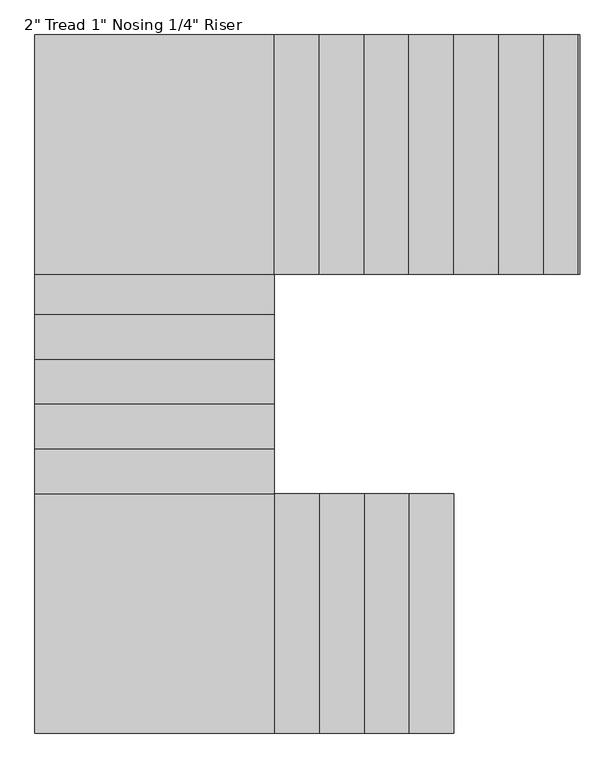
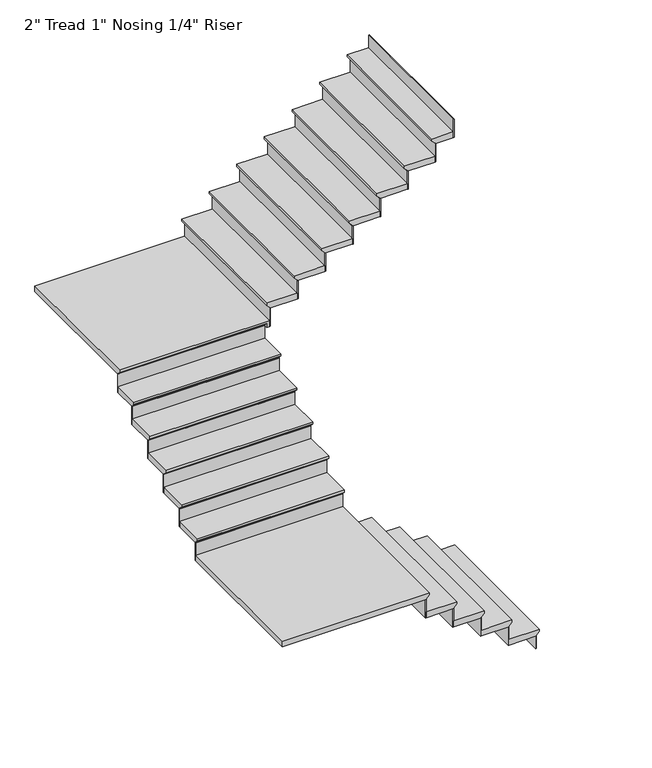
"""IFC4 building model written with IfcOpenShell, lengths in millimetres: stair flight geometry."""

from ifc_helpers import new_model, si_unit, origin, place, context, project, spatial, faceted_brep, source, transform, mapped, element, save


def stair_flight_7559bbc3(model_context):
    return source(origin(), model_context, "Body", "Brep", [
        faceted_brep([(-2683.1105391, -1521.8373761, 3189.3710526), (-2683.1105391, -1521.8373761, 3208.4210526), (-2683.1105391, -2741.0373761, 3208.4210526), (-2683.1105391, -2741.0373761, 3189.3710526), (-2708.5105391, -1521.8373761, 3163.9710526), (-2708.5105391, -2741.0373761, 3163.9710526), (-2937.1105391, -1521.8373761, 3208.4210526), (-2937.1105391, -2741.0373761, 3208.4210526), (-2708.5105391, -2741.0373761, 3157.6210526), (-2937.1105391, -2741.0373761, 3157.6210526), (-2937.1105391, -1521.8373761, 3157.6210526), (-2708.5105391, -1521.8373761, 3157.6210526)], [[[0, 1, 2, 3]], [[4, 0, 3, 5]], [[2, 1, 6, 7]], [[8, 9, 10, 11]], [[2, 7, 9, 8, 5, 3]], [[8, 11, 4, 5]], [[6, 1, 0, 4, 11, 10]], [[7, 6, 10, 9]]]),
        faceted_brep([(-2708.5105391, -1521.8373761, 3157.6210526), (-2708.5105391, -1521.8373761, 3048.0), (-2714.8605391, -1521.8373761, 3048.0), (-2714.8605391, -1521.8373761, 3157.6210526), (-2708.5105391, -2741.0373761, 3157.6210526), (-2714.8605391, -2741.0373761, 3157.6210526), (-2714.8605391, -2741.0373761, 3048.0), (-2708.5105391, -2741.0373761, 3048.0)], [[[0, 1, 2, 3]], [[4, 5, 6, 7]], [[1, 0, 4, 7]], [[2, 1, 7, 6]], [[3, 2, 6, 5]], [[0, 3, 5, 4]]]),
        faceted_brep([(-2937.1105391, -1521.8373761, 3318.0421053), (-2937.1105391, -1521.8373761, 3157.6210526), (-2943.4605391, -1521.8373761, 3157.6210526), (-2943.4605391, -1521.8373761, 3318.0421053), (-2937.1105391, -2741.0373761, 3318.0421053), (-2943.4605391, -2741.0373761, 3318.0421053), (-2943.4605391, -2741.0373761, 3157.6210526), (-2937.1105391, -2741.0373761, 3157.6210526)], [[[0, 1, 2, 3]], [[4, 5, 6, 7]], [[1, 0, 4, 7]], [[2, 1, 7, 6]], [[3, 2, 6, 5]], [[0, 3, 5, 4]]]),
        faceted_brep([(-2911.7105391, -2741.0373761, 3368.8421053), (-2911.7105391, -1521.8373761, 3368.8421053), (-3165.7105391, -1521.8373761, 3368.8421053), (-3165.7105391, -2741.0373761, 3368.8421053), (-2937.1105391, -2741.0373761, 3318.0421053), (-3165.7105391, -2741.0373761, 3318.0421053), (-3165.7105391, -1521.8373761, 3318.0421053), (-2937.1105391, -1521.8373761, 3318.0421053), (-2937.1105391, -2741.0373761, 3324.3921053), (-2911.7105391, -2741.0373761, 3349.7921053), (-2937.1105391, -1521.8373761, 3324.3921053), (-2911.7105391, -1521.8373761, 3349.7921053)], [[[0, 1, 2, 3]], [[4, 5, 6, 7]], [[0, 3, 5, 4, 8, 9]], [[4, 7, 10, 8]], [[2, 1, 11, 10, 7, 6]], [[3, 2, 6, 5]], [[11, 1, 0, 9]], [[10, 11, 9, 8]]]),
        faceted_brep([(-3165.7105391, -1521.8373761, 3478.4631579), (-3165.7105391, -1521.8373761, 3318.0421053), (-3172.0605391, -1521.8373761, 3318.0421053), (-3172.0605391, -1521.8373761, 3478.4631579), (-3165.7105391, -2741.0373761, 3478.4631579), (-3172.0605391, -2741.0373761, 3478.4631579), (-3172.0605391, -2741.0373761, 3318.0421053), (-3165.7105391, -2741.0373761, 3318.0421053)], [[[0, 1, 2, 3]], [[4, 5, 6, 7]], [[1, 0, 4, 7]], [[2, 1, 7, 6]], [[3, 2, 6, 5]], [[0, 3, 5, 4]]]),
        faceted_brep([(-3140.3105391, -2741.0373761, 3529.2631579), (-3140.3105391, -1521.8373761, 3529.2631579), (-3394.3105391, -1521.8373761, 3529.2631579), (-3394.3105391, -2741.0373761, 3529.2631579), (-3165.7105391, -2741.0373761, 3478.4631579), (-3394.3105391, -2741.0373761, 3478.4631579), (-3394.3105391, -1521.8373761, 3478.4631579), (-3165.7105391, -1521.8373761, 3478.4631579), (-3165.7105391, -2741.0373761, 3484.8131579), (-3140.3105391, -2741.0373761, 3510.2131579), (-3165.7105391, -1521.8373761, 3484.8131579), (-3140.3105391, -1521.8373761, 3510.2131579)], [[[0, 1, 2, 3]], [[4, 5, 6, 7]], [[0, 3, 5, 4, 8, 9]], [[4, 7, 10, 8]], [[2, 1, 11, 10, 7, 6]], [[3, 2, 6, 5]], [[11, 1, 0, 9]], [[10, 11, 9, 8]]]),
        faceted_brep([(-3394.3105391, -1521.8373761, 3638.8842105), (-3394.3105391, -1521.8373761, 3478.4631579), (-3400.6605391, -1521.8373761, 3478.4631579), (-3400.6605391, -1521.8373761, 3638.8842105), (-3394.3105391, -2741.0373761, 3638.8842105), (-3400.6605391, -2741.0373761, 3638.8842105), (-3400.6605391, -2741.0373761, 3478.4631579), (-3394.3105391, -2741.0373761, 3478.4631579)], [[[0, 1, 2, 3]], [[4, 5, 6, 7]], [[1, 0, 4, 7]], [[2, 1, 7, 6]], [[3, 2, 6, 5]], [[0, 3, 5, 4]]]),
        faceted_brep([(-3368.9105391, -2741.0373761, 3689.6842105), (-3368.9105391, -1521.8373761, 3689.6842105), (-3622.9105391, -1521.8373761, 3689.6842105), (-3622.9105391, -2741.0373761, 3689.6842105), (-3394.3105391, -2741.0373761, 3638.8842105), (-3622.9105391, -2741.0373761, 3638.8842105), (-3622.9105391, -1521.8373761, 3638.8842105), (-3394.3105391, -1521.8373761, 3638.8842105), (-3394.3105391, -2741.0373761, 3645.2342105), (-3368.9105391, -2741.0373761, 3670.6342105), (-3394.3105391, -1521.8373761, 3645.2342105), (-3368.9105391, -1521.8373761, 3670.6342105)], [[[0, 1, 2, 3]], [[4, 5, 6, 7]], [[0, 3, 5, 4, 8, 9]], [[4, 7, 10, 8]], [[2, 1, 11, 10, 7, 6]], [[3, 2, 6, 5]], [[11, 1, 0, 9]], [[10, 11, 9, 8]]]),
        faceted_brep([(-3622.9105391, -1521.8373761, 3799.3052632), (-3622.9105391, -1521.8373761, 3638.8842105), (-3629.2605391, -1521.8373761, 3638.8842105), (-3629.2605391, -1521.8373761, 3799.3052632), (-3622.9105391, -2741.0373761, 3799.3052632), (-3629.2605391, -2741.0373761, 3799.3052632), (-3629.2605391, -2741.0373761, 3638.8842105), (-3622.9105391, -2741.0373761, 3638.8842105)], [[[0, 1, 2, 3]], [[4, 5, 6, 7]], [[1, 0, 4, 7]], [[2, 1, 7, 6]], [[3, 2, 6, 5]], [[0, 3, 5, 4]]]),
        faceted_brep([(-4816.7105391, -1496.4373761, 3850.1052632), (-4816.7105391, -2741.0373761, 3850.1052632), (-3597.5105391, -2741.0373761, 3850.1052632), (-3597.5105391, -1496.4373761, 3850.1052632), (-4816.7105391, -2741.0373761, 3799.3052632), (-4816.7105391, -1496.4373761, 3799.3052632), (-3597.5105391, -1496.4373761, 3799.3052632), (-3597.5105391, -1521.8373761, 3799.3052632), (-3622.9105391, -1521.8373761, 3799.3052632), (-3622.9105391, -2741.0373761, 3799.3052632), (-3622.9105391, -2741.0373761, 3805.6552632), (-3597.5105391, -2741.0373761, 3831.0552632), (-3622.9105391, -1521.8373761, 3805.6552632), (-3597.5105391, -1521.8373761, 3831.0552632)], [[[0, 1, 2, 3]], [[4, 5, 6, 7, 8, 9]], [[1, 0, 5, 4]], [[2, 1, 4, 9, 10, 11]], [[9, 8, 12, 10]], [[8, 7, 13, 12]], [[3, 2, 11, 13, 7, 6]], [[0, 3, 6, 5]], [[11, 10, 12, 13]]]),
        faceted_brep([(-3597.5105391, -1496.4373761, 3959.7263158), (-3597.5105391, -1496.4373761, 3799.3052632), (-3597.5105391, -1490.0873761, 3799.3052632), (-3597.5105391, -1490.0873761, 3959.7263158), (-4816.7105391, -1496.4373761, 3959.7263158), (-4816.7105391, -1490.0873761, 3959.7263158), (-4816.7105391, -1490.0873761, 3799.3052632), (-4816.7105391, -1496.4373761, 3799.3052632)], [[[0, 1, 2, 3]], [[4, 5, 6, 7]], [[1, 0, 4, 7]], [[2, 1, 7, 6]], [[3, 2, 6, 5]], [[0, 3, 5, 4]]]),
        faceted_brep([(-4816.7105391, -1521.8373761, 4010.5263158), (-3597.5105391, -1521.8373761, 4010.5263158), (-3597.5105391, -1267.8373761, 4010.5263158), (-4816.7105391, -1267.8373761, 4010.5263158), (-4816.7105391, -1496.4373761, 3959.7263158), (-4816.7105391, -1267.8373761, 3959.7263158), (-3597.5105391, -1267.8373761, 3959.7263158), (-3597.5105391, -1496.4373761, 3959.7263158), (-4816.7105391, -1496.4373761, 3966.0763158), (-4816.7105391, -1521.8373761, 3991.4763158), (-3597.5105391, -1496.4373761, 3966.0763158), (-3597.5105391, -1521.8373761, 3991.4763158)], [[[0, 1, 2, 3]], [[4, 5, 6, 7]], [[0, 3, 5, 4, 8, 9]], [[4, 7, 10, 8]], [[2, 1, 11, 10, 7, 6]], [[3, 2, 6, 5]], [[11, 1, 0, 9]], [[10, 11, 9, 8]]]),
        faceted_brep([(-3597.5105391, -1267.8373761, 4120.1473684), (-3597.5105391, -1267.8373761, 3959.7263158), (-3597.5105391, -1261.4873761, 3959.7263158), (-3597.5105391, -1261.4873761, 4120.1473684), (-4816.7105391, -1267.8373761, 4120.1473684), (-4816.7105391, -1261.4873761, 4120.1473684), (-4816.7105391, -1261.4873761, 3959.7263158), (-4816.7105391, -1267.8373761, 3959.7263158)], [[[0, 1, 2, 3]], [[4, 5, 6, 7]], [[1, 0, 4, 7]], [[2, 1, 7, 6]], [[3, 2, 6, 5]], [[0, 3, 5, 4]]]),
        faceted_brep([(-4816.7105391, -1293.2373761, 4170.9473684), (-3597.5105391, -1293.2373761, 4170.9473684), (-3597.5105391, -1039.2373761, 4170.9473684), (-4816.7105391, -1039.2373761, 4170.9473684), (-4816.7105391, -1267.8373761, 4120.1473684), (-4816.7105391, -1039.2373761, 4120.1473684), (-3597.5105391, -1039.2373761, 4120.1473684), (-3597.5105391, -1267.8373761, 4120.1473684), (-4816.7105391, -1267.8373761, 4126.4973684), (-4816.7105391, -1293.2373761, 4151.8973684), (-3597.5105391, -1267.8373761, 4126.4973684), (-3597.5105391, -1293.2373761, 4151.8973684)], [[[0, 1, 2, 3]], [[4, 5, 6, 7]], [[0, 3, 5, 4, 8, 9]], [[4, 7, 10, 8]], [[2, 1, 11, 10, 7, 6]], [[3, 2, 6, 5]], [[11, 1, 0, 9]], [[10, 11, 9, 8]]]),
        faceted_brep([(-3597.5105391, -1039.2373761, 4280.5684211), (-3597.5105391, -1039.2373761, 4120.1473684), (-3597.5105391, -1032.8873761, 4120.1473684), (-3597.5105391, -1032.8873761, 4280.5684211), (-4816.7105391, -1039.2373761, 4280.5684211), (-4816.7105391, -1032.8873761, 4280.5684211), (-4816.7105391, -1032.8873761, 4120.1473684), (-4816.7105391, -1039.2373761, 4120.1473684)], [[[0, 1, 2, 3]], [[4, 5, 6, 7]], [[1, 0, 4, 7]], [[2, 1, 7, 6]], [[3, 2, 6, 5]], [[0, 3, 5, 4]]]),
        faceted_brep([(-4816.7105391, -1064.6373761, 4331.3684211), (-3597.5105391, -1064.6373761, 4331.3684211), (-3597.5105391, -810.6373761, 4331.3684211), (-4816.7105391, -810.6373761, 4331.3684211), (-4816.7105391, -1039.2373761, 4280.5684211), (-4816.7105391, -810.6373761, 4280.5684211), (-3597.5105391, -810.6373761, 4280.5684211), (-3597.5105391, -1039.2373761, 4280.5684211), (-4816.7105391, -1039.2373761, 4286.9184211), (-4816.7105391, -1064.6373761, 4312.3184211), (-3597.5105391, -1039.2373761, 4286.9184211), (-3597.5105391, -1064.6373761, 4312.3184211)], [[[0, 1, 2, 3]], [[4, 5, 6, 7]], [[0, 3, 5, 4, 8, 9]], [[4, 7, 10, 8]], [[2, 1, 11, 10, 7, 6]], [[3, 2, 6, 5]], [[11, 1, 0, 9]], [[10, 11, 9, 8]]]),
        faceted_brep([(-3597.5105391, -810.6373761, 4440.9894737), (-3597.5105391, -810.6373761, 4280.5684211), (-3597.5105391, -804.2873761, 4280.5684211), (-3597.5105391, -804.2873761, 4440.9894737), (-4816.7105391, -810.6373761, 4440.9894737), (-4816.7105391, -804.2873761, 4440.9894737), (-4816.7105391, -804.2873761, 4280.5684211), (-4816.7105391, -810.6373761, 4280.5684211)], [[[0, 1, 2, 3]], [[4, 5, 6, 7]], [[1, 0, 4, 7]], [[2, 1, 7, 6]], [[3, 2, 6, 5]], [[0, 3, 5, 4]]]),
        faceted_brep([(-4816.7105391, -836.0373761, 4491.7894737), (-3597.5105391, -836.0373761, 4491.7894737), (-3597.5105391, -582.0373761, 4491.7894737), (-4816.7105391, -582.0373761, 4491.7894737), (-4816.7105391, -810.6373761, 4440.9894737), (-4816.7105391, -582.0373761, 4440.9894737), (-3597.5105391, -582.0373761, 4440.9894737), (-3597.5105391, -810.6373761, 4440.9894737), (-4816.7105391, -810.6373761, 4447.3394737), (-4816.7105391, -836.0373761, 4472.7394737), (-3597.5105391, -810.6373761, 4447.3394737), (-3597.5105391, -836.0373761, 4472.7394737)], [[[0, 1, 2, 3]], [[4, 5, 6, 7]], [[0, 3, 5, 4, 8, 9]], [[4, 7, 10, 8]], [[2, 1, 11, 10, 7, 6]], [[3, 2, 6, 5]], [[11, 1, 0, 9]], [[10, 11, 9, 8]]]),
        faceted_brep([(-3597.5105391, -582.0373761, 4601.4105263), (-3597.5105391, -582.0373761, 4440.9894737), (-3597.5105391, -575.6873761, 4440.9894737), (-3597.5105391, -575.6873761, 4601.4105263), (-4816.7105391, -582.0373761, 4601.4105263), (-4816.7105391, -575.6873761, 4601.4105263), (-4816.7105391, -575.6873761, 4440.9894737), (-4816.7105391, -582.0373761, 4440.9894737)], [[[0, 1, 2, 3]], [[4, 5, 6, 7]], [[1, 0, 4, 7]], [[2, 1, 7, 6]], [[3, 2, 6, 5]], [[0, 3, 5, 4]]]),
        faceted_brep([(-4816.7105391, -607.4373761, 4652.2105263), (-3597.5105391, -607.4373761, 4652.2105263), (-3597.5105391, -378.8373761, 4652.2105263), (-4816.7105391, -378.8373761, 4652.2105263), (-4816.7105391, -582.0373761, 4601.4105263), (-4816.7105391, -378.8373761, 4601.4105263), (-3597.5105391, -378.8373761, 4601.4105263), (-3597.5105391, -582.0373761, 4601.4105263), (-4816.7105391, -582.0373761, 4607.7605263), (-4816.7105391, -607.4373761, 4633.1605263), (-3597.5105391, -582.0373761, 4607.7605263), (-3597.5105391, -607.4373761, 4633.1605263)], [[[0, 1, 2, 3]], [[4, 5, 6, 7]], [[0, 3, 5, 4, 8, 9]], [[4, 7, 10, 8]], [[2, 1, 11, 10, 7, 6]], [[3, 2, 6, 5]], [[11, 1, 0, 9]], [[10, 11, 9, 8]]]),
        faceted_brep([(-3597.5105391, -378.8373761, 4761.8315789), (-3597.5105391, -378.8373761, 4601.4105263), (-3597.5105391, -372.4873761, 4601.4105263), (-3597.5105391, -372.4873761, 4761.8315789), (-4816.7105391, -378.8373761, 4761.8315789), (-4816.7105391, -372.4873761, 4761.8315789), (-4816.7105391, -372.4873761, 4601.4105263), (-4816.7105391, -378.8373761, 4601.4105263)], [[[0, 1, 2, 3]], [[4, 5, 6, 7]], [[1, 0, 4, 7]], [[2, 1, 7, 6]], [[3, 2, 6, 5]], [[0, 3, 5, 4]]]),
        faceted_brep([(-3572.1105391, 814.9626239, 4812.6315789), (-4816.7105391, 814.9626239, 4812.6315789), (-4816.7105391, -404.2373761, 4812.6315789), (-3572.1105391, -404.2373761, 4812.6315789), (-4816.7105391, 814.9626239, 4761.8315789), (-3572.1105391, 814.9626239, 4761.8315789), (-3572.1105391, -404.2373761, 4761.8315789), (-3597.5105391, -404.2373761, 4761.8315789), (-3597.5105391, -378.8373761, 4761.8315789), (-4816.7105391, -378.8373761, 4761.8315789), (-4816.7105391, -378.8373761, 4768.1815789), (-4816.7105391, -404.2373761, 4793.5815789), (-3597.5105391, -378.8373761, 4768.1815789), (-3597.5105391, -404.2373761, 4793.5815789)], [[[0, 1, 2, 3]], [[4, 5, 6, 7, 8, 9]], [[1, 0, 5, 4]], [[2, 1, 4, 9, 10, 11]], [[9, 8, 12, 10]], [[8, 7, 13, 12]], [[3, 2, 11, 13, 7, 6]], [[0, 3, 6, 5]], [[11, 10, 12, 13]]]),
        faceted_brep([(-3572.1105391, -404.2373761, 4922.2526316), (-3572.1105391, -404.2373761, 4761.8315789), (-3565.7605391, -404.2373761, 4761.8315789), (-3565.7605391, -404.2373761, 4922.2526316), (-3572.1105391, 814.9626239, 4922.2526316), (-3565.7605391, 814.9626239, 4922.2526316), (-3565.7605391, 814.9626239, 4761.8315789), (-3572.1105391, 814.9626239, 4761.8315789)], [[[0, 1, 2, 3]], [[4, 5, 6, 7]], [[1, 0, 4, 7]], [[2, 1, 7, 6]], [[3, 2, 6, 5]], [[0, 3, 5, 4]]]),
        faceted_brep([(-3597.5105391, 814.9626239, 4973.0526316), (-3597.5105391, -404.2373761, 4973.0526316), (-3343.5105391, -404.2373761, 4973.0526316), (-3343.5105391, 814.9626239, 4973.0526316), (-3572.1105391, 814.9626239, 4922.2526316), (-3343.5105391, 814.9626239, 4922.2526316), (-3343.5105391, -404.2373761, 4922.2526316), (-3572.1105391, -404.2373761, 4922.2526316), (-3572.1105391, 814.9626239, 4928.6026316), (-3597.5105391, 814.9626239, 4954.0026316), (-3572.1105391, -404.2373761, 4928.6026316), (-3597.5105391, -404.2373761, 4954.0026316)], [[[0, 1, 2, 3]], [[4, 5, 6, 7]], [[0, 3, 5, 4, 8, 9]], [[4, 7, 10, 8]], [[2, 1, 11, 10, 7, 6]], [[3, 2, 6, 5]], [[11, 1, 0, 9]], [[10, 11, 9, 8]]]),
        faceted_brep([(-3343.5105391, -404.2373761, 5082.6736842), (-3343.5105391, -404.2373761, 4922.2526316), (-3337.1605391, -404.2373761, 4922.2526316), (-3337.1605391, -404.2373761, 5082.6736842), (-3343.5105391, 814.9626239, 5082.6736842), (-3337.1605391, 814.9626239, 5082.6736842), (-3337.1605391, 814.9626239, 4922.2526316), (-3343.5105391, 814.9626239, 4922.2526316)], [[[0, 1, 2, 3]], [[4, 5, 6, 7]], [[1, 0, 4, 7]], [[2, 1, 7, 6]], [[3, 2, 6, 5]], [[0, 3, 5, 4]]]),
        faceted_brep([(-3368.9105391, 814.9626239, 5133.4736842), (-3368.9105391, -404.2373761, 5133.4736842), (-3114.9105391, -404.2373761, 5133.4736842), (-3114.9105391, 814.9626239, 5133.4736842), (-3343.5105391, 814.9626239, 5082.6736842), (-3114.9105391, 814.9626239, 5082.6736842), (-3114.9105391, -404.2373761, 5082.6736842), (-3343.5105391, -404.2373761, 5082.6736842), (-3343.5105391, 814.9626239, 5089.0236842), (-3368.9105391, 814.9626239, 5114.4236842), (-3343.5105391, -404.2373761, 5089.0236842), (-3368.9105391, -404.2373761, 5114.4236842)], [[[0, 1, 2, 3]], [[4, 5, 6, 7]], [[0, 3, 5, 4, 8, 9]], [[4, 7, 10, 8]], [[2, 1, 11, 10, 7, 6]], [[3, 2, 6, 5]], [[11, 1, 0, 9]], [[10, 11, 9, 8]]]),
        faceted_brep([(-3114.9105391, -404.2373761, 5243.0947368), (-3114.9105391, -404.2373761, 5082.6736842), (-3108.5605391, -404.2373761, 5082.6736842), (-3108.5605391, -404.2373761, 5243.0947368), (-3114.9105391, 814.9626239, 5243.0947368), (-3108.5605391, 814.9626239, 5243.0947368), (-3108.5605391, 814.9626239, 5082.6736842), (-3114.9105391, 814.9626239, 5082.6736842)], [[[0, 1, 2, 3]], [[4, 5, 6, 7]], [[1, 0, 4, 7]], [[2, 1, 7, 6]], [[3, 2, 6, 5]], [[0, 3, 5, 4]]]),
        faceted_brep([(-3140.3105391, 814.9626239, 5293.8947368), (-3140.3105391, -404.2373761, 5293.8947368), (-2886.3105391, -404.2373761, 5293.8947368), (-2886.3105391, 814.9626239, 5293.8947368), (-3114.9105391, 814.9626239, 5243.0947368), (-2886.3105391, 814.9626239, 5243.0947368), (-2886.3105391, -404.2373761, 5243.0947368), (-3114.9105391, -404.2373761, 5243.0947368), (-3114.9105391, 814.9626239, 5249.4447368), (-3140.3105391, 814.9626239, 5274.8447368), (-3114.9105391, -404.2373761, 5249.4447368), (-3140.3105391, -404.2373761, 5274.8447368)], [[[0, 1, 2, 3]], [[4, 5, 6, 7]], [[0, 3, 5, 4, 8, 9]], [[4, 7, 10, 8]], [[2, 1, 11, 10, 7, 6]], [[3, 2, 6, 5]], [[11, 1, 0, 9]], [[10, 11, 9, 8]]]),
        faceted_brep([(-2886.3105391, -404.2373761, 5403.5157895), (-2886.3105391, -404.2373761, 5243.0947368), (-2879.9605391, -404.2373761, 5243.0947368), (-2879.9605391, -404.2373761, 5403.5157895), (-2886.3105391, 814.9626239, 5403.5157895), (-2879.9605391, 814.9626239, 5403.5157895), (-2879.9605391, 814.9626239, 5243.0947368), (-2886.3105391, 814.9626239, 5243.0947368)], [[[0, 1, 2, 3]], [[4, 5, 6, 7]], [[1, 0, 4, 7]], [[2, 1, 7, 6]], [[3, 2, 6, 5]], [[0, 3, 5, 4]]]),
        faceted_brep([(-2911.7105391, 814.9626239, 5454.3157895), (-2911.7105391, -404.2373761, 5454.3157895), (-2657.7105391, -404.2373761, 5454.3157895), (-2657.7105391, 814.9626239, 5454.3157895), (-2886.3105391, 814.9626239, 5403.5157895), (-2657.7105391, 814.9626239, 5403.5157895), (-2657.7105391, -404.2373761, 5403.5157895), (-2886.3105391, -404.2373761, 5403.5157895), (-2886.3105391, 814.9626239, 5409.8657895), (-2911.7105391, 814.9626239, 5435.2657895), (-2886.3105391, -404.2373761, 5409.8657895), (-2911.7105391, -404.2373761, 5435.2657895)], [[[0, 1, 2, 3]], [[4, 5, 6, 7]], [[0, 3, 5, 4, 8, 9]], [[4, 7, 10, 8]], [[2, 1, 11, 10, 7, 6]], [[3, 2, 6, 5]], [[11, 1, 0, 9]], [[10, 11, 9, 8]]]),
        faceted_brep([(-2657.7105391, -404.2373761, 5563.9368421), (-2657.7105391, -404.2373761, 5403.5157895), (-2651.3605391, -404.2373761, 5403.5157895), (-2651.3605391, -404.2373761, 5563.9368421), (-2657.7105391, 814.9626239, 5563.9368421), (-2651.3605391, 814.9626239, 5563.9368421), (-2651.3605391, 814.9626239, 5403.5157895), (-2657.7105391, 814.9626239, 5403.5157895)], [[[0, 1, 2, 3]], [[4, 5, 6, 7]], [[1, 0, 4, 7]], [[2, 1, 7, 6]], [[3, 2, 6, 5]], [[0, 3, 5, 4]]]),
        faceted_brep([(-2683.1105391, 814.9626239, 5614.7368421), (-2683.1105391, -404.2373761, 5614.7368421), (-2429.1105391, -404.2373761, 5614.7368421), (-2429.1105391, 814.9626239, 5614.7368421), (-2657.7105391, 814.9626239, 5563.9368421), (-2429.1105391, 814.9626239, 5563.9368421), (-2429.1105391, -404.2373761, 5563.9368421), (-2657.7105391, -404.2373761, 5563.9368421), (-2657.7105391, 814.9626239, 5570.2868421), (-2683.1105391, 814.9626239, 5595.6868421), (-2657.7105391, -404.2373761, 5570.2868421), (-2683.1105391, -404.2373761, 5595.6868421)], [[[0, 1, 2, 3]], [[4, 5, 6, 7]], [[0, 3, 5, 4, 8, 9]], [[4, 7, 10, 8]], [[2, 1, 11, 10, 7, 6]], [[3, 2, 6, 5]], [[11, 1, 0, 9]], [[10, 11, 9, 8]]]),
        faceted_brep([(-2429.1105391, -404.2373761, 5724.3578947), (-2429.1105391, -404.2373761, 5563.9368421), (-2422.7605391, -404.2373761, 5563.9368421), (-2422.7605391, -404.2373761, 5724.3578947), (-2429.1105391, 814.9626239, 5724.3578947), (-2422.7605391, 814.9626239, 5724.3578947), (-2422.7605391, 814.9626239, 5563.9368421), (-2429.1105391, 814.9626239, 5563.9368421)], [[[0, 1, 2, 3]], [[4, 5, 6, 7]], [[1, 0, 4, 7]], [[2, 1, 7, 6]], [[3, 2, 6, 5]], [[0, 3, 5, 4]]]),
        faceted_brep([(-2454.5105391, 814.9626239, 5775.1578947), (-2454.5105391, -404.2373761, 5775.1578947), (-2200.5105391, -404.2373761, 5775.1578947), (-2200.5105391, 814.9626239, 5775.1578947), (-2429.1105391, 814.9626239, 5724.3578947), (-2200.5105391, 814.9626239, 5724.3578947), (-2200.5105391, -404.2373761, 5724.3578947), (-2429.1105391, -404.2373761, 5724.3578947), (-2429.1105391, 814.9626239, 5730.7078947), (-2454.5105391, 814.9626239, 5756.1078947), (-2429.1105391, -404.2373761, 5730.7078947), (-2454.5105391, -404.2373761, 5756.1078947)], [[[0, 1, 2, 3]], [[4, 5, 6, 7]], [[0, 3, 5, 4, 8, 9]], [[4, 7, 10, 8]], [[2, 1, 11, 10, 7, 6]], [[3, 2, 6, 5]], [[11, 1, 0, 9]], [[10, 11, 9, 8]]]),
        faceted_brep([(-2200.5105391, -404.2373761, 5884.7789474), (-2200.5105391, -404.2373761, 5724.3578947), (-2194.1605391, -404.2373761, 5724.3578947), (-2194.1605391, -404.2373761, 5884.7789474), (-2200.5105391, 814.9626239, 5884.7789474), (-2194.1605391, 814.9626239, 5884.7789474), (-2194.1605391, 814.9626239, 5724.3578947), (-2200.5105391, 814.9626239, 5724.3578947)], [[[0, 1, 2, 3]], [[4, 5, 6, 7]], [[1, 0, 4, 7]], [[2, 1, 7, 6]], [[3, 2, 6, 5]], [[0, 3, 5, 4]]]),
        faceted_brep([(-2048.1105391, -404.2373761, 6045.2), (-2048.1105391, -404.2373761, 5884.7789474), (-2041.7605391, -404.2373761, 5884.7789474), (-2041.7605391, -404.2373761, 6045.2), (-2048.1105391, 814.9626239, 6045.2), (-2041.7605391, 814.9626239, 6045.2), (-2041.7605391, 814.9626239, 5884.7789474), (-2048.1105391, 814.9626239, 5884.7789474)], [[[0, 1, 2, 3]], [[4, 5, 6, 7]], [[1, 0, 4, 7]], [[2, 1, 7, 6]], [[3, 2, 6, 5]], [[0, 3, 5, 4]]]),
        faceted_brep([(-2225.9105391, 814.9626239, 5935.5789474), (-2225.9105391, -404.2373761, 5935.5789474), (-2048.1105391, -404.2373761, 5935.5789474), (-2048.1105391, 814.9626239, 5935.5789474), (-2200.5105391, 814.9626239, 5884.7789474), (-2048.1105391, 814.9626239, 5884.7789474), (-2048.1105391, -404.2373761, 5884.7789474), (-2200.5105391, -404.2373761, 5884.7789474), (-2200.5105391, 814.9626239, 5891.1289474), (-2225.9105391, 814.9626239, 5916.5289474), (-2200.5105391, -404.2373761, 5891.1289474), (-2225.9105391, -404.2373761, 5916.5289474)], [[[0, 1, 2, 3]], [[4, 5, 6, 7]], [[0, 3, 5, 4, 8, 9]], [[4, 7, 10, 8]], [[2, 1, 11, 10, 7, 6]], [[3, 2, 6, 5]], [[11, 1, 0, 9]], [[10, 11, 9, 8]]]),
    ])


if __name__ == "__main__":
    model = new_model("IFC4")
    model_context = context("Model", 3, world=origin())
    ifc_project = project(units=[si_unit("LENGTHUNIT", "METRE", prefix="MILLI")], contexts=[model_context])
    site = spatial("IfcSite", under=ifc_project)
    building = spatial("IfcBuilding", under=site)
    placement = place(None, origin())
    stair_flight_shape = stair_flight_7559bbc3(model_context)
    element("IfcStairFlight", 1, ObjectType="2\" Tread 1\" Nosing 1/4\" Riser", at=placement, inside=building, context=model_context, shape_type="MappedRepresentation", body=[
        mapped(stair_flight_shape, transform((0.0, 0.0, 0.0), x_axis=(1.0, 0.0, 0.0), y_axis=(0.0, 1.0, 0.0), z_axis=(0.0, 0.0, 1.0))),
    ])
    save(model, "model.ifc")
